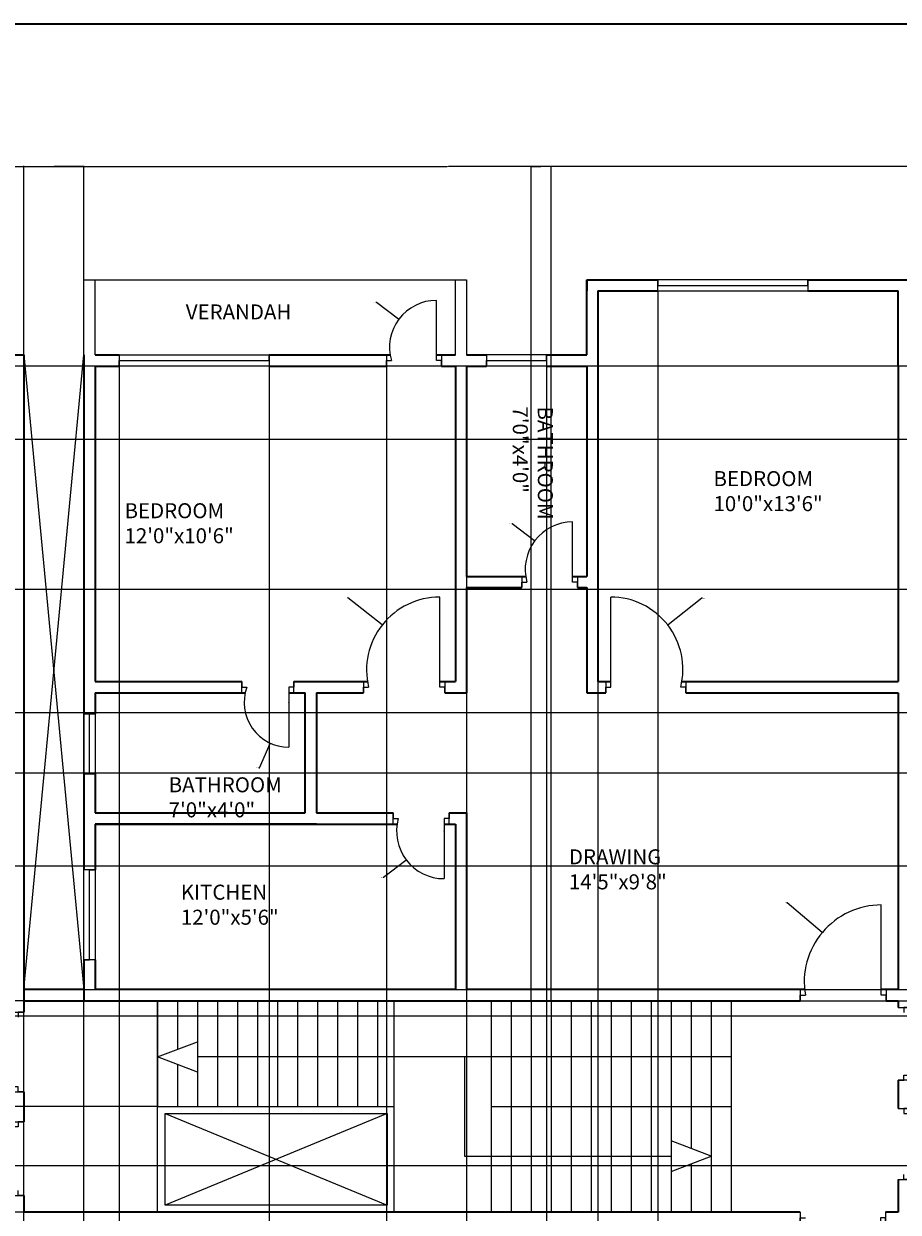
# Model space of a CAD drawing. Units: inches. Extents: x 1831 to 2867, y 1605 to 2524.
# Tile 5 of 7: x 2172 to 2522, y 2049 to 2524. Entities that reach past the tile are written whole.
import ezdxf

# ---------------------------------------------------------------- set-up
doc = ezdxf.new("R2010")
doc.units = ezdxf.units.IN
for name, color, linetype, lineweight in [('A-ANNO-DIMS', 2, 'Continuous', 18), ('A-ANNO-SYMB', 81, 'Continuous', 18), ('A-ANNO-TTLB', 7, 'Continuous', 35), ('A-AREA-IDEN', 7, 'Continuous', 18), ('A-DOOR', 11, 'Continuous', 18), ('A-FLOR-BALC', 7, 'Continuous', 25), ('A-FLOR-OPEN', 7, 'Continuous', 13), ('A-FLOR-STRS', 81, 'Continuous', 18), ('A-GLAZ', 121, 'Continuous', 18), ('A-WALL', 7, 'Continuous', 35)]:
    doc.layers.add(name, color=color, linetype=linetype, lineweight=lineweight)
doc.styles.get("Standard").update_dxf_attribs({"font": 'arial.ttf'})
doc.dimstyles.get("Standard").update_dxf_attribs({"dimtxt": 0.18, "dimasz": 0.18, "dimexe": 0.18, "dimexo": 0.0625, "dimgap": 0.09, "dimtad": 0, "dimtih": 1, "dimtoh": 1, "dimdec": 4, "dimzin": 0, "dimdsep": 46, "dimtxsty": 'Standard', "dimcen": 0.09, "dimadec": 0, "dimazin": 0, "dimtfac": 1, "dimtdec": 4, "dimtofl": 0, "dimtmove": 0, "dimatfit": 3, "dimfxl": 1, "dimtolj": 1, "dimtzin": 0, "dimarcsym": 0})

# ---------------------------------------------------------------- blocks, each defined once
blk = doc.blocks.new('WIN-60IN')
for p, q in [((4.5, 60), (0, 60)), ((0, 60), (2.25, 60)), ((0, 0), (0, 60)), ((2.25, 60), (2.25, 0)), ((4.5, 60), (4.5, 0)), ((4.5, 0), (0, 0)), ((2.25, 0), (4.5, 0))]:
    blk.add_line(p, q)
blk = doc.blocks.new('WIN-24IN')
for p, q in [((4.5, 24), (0, 24)), ((0, 24), (2.25, 24)), ((0, 0), (0, 24)), ((2.25, 24), (2.25, 0)), ((4.5, 0), (4.5, 24)), ((4.5, 0), (0, 0)), ((2.25, 0), (4.5, 0))]:
    blk.add_line(p, q)
blk = doc.blocks.new('WIN-36IN')
for p, q in [((0, 0), (0, 4.5)), ((36, 4.5), (0, 4.5)), ((36, 2.25), (0, 2.25)), ((0, 2.25), (0, 0)), ((36, 0), (36, 4.5)), ((36, 4.5), (36, 2.25)), ((0, 0), (36, 0))]:
    blk.add_line(p, q)
blk = doc.blocks.new('WIN-60IN-ALT')
for p, q in [((0, 0), (0, 4.5)), ((0, 4.5), (0, 2.25)), ((60, 4.5), (0, 4.5)), ((0, 2.25), (60, 2.25)), ((0, 0), (60, 0)), ((60, 2.25), (60, 4.5)), ((60, 4.5), (60, 0))]:
    blk.add_line(p, q)
blk = doc.blocks.new('DOOR-LEAF-36IN')
for p, q in [((0, 2), (4.5, 2)), ((4.5, 2), (2.25, 2)), ((2.25, 2), (2.25, 0)), ((2.25, 0), (38.25, 0))]:
    blk.add_line(p, q)
blk = doc.blocks.new('DOOR-LEAF-36IN-ALT')
for p, q in [((36, 2), (0, 2)), ((33.75, 0), (38.25, 0)), ((36, 0), (36, 2)), ((38.25, 0), (36, 0))]:
    blk.add_line(p, q)
blk = doc.blocks.new('DOOR-LEAF-24IN-ALT')
for p, q in [((24, 2), (0, 2)), ((21.75, 0), (26.25, 0)), ((24, 0), (24, 2)), ((26.25, 0), (24, 0))]:
    blk.add_line(p, q)
blk = doc.blocks.new('DOOR-STRIKE-JAMB')
for p, q in [((0, 0), (4.5, 0)), ((2.25, 0), (2.25, 2)), ((4.5, 0), (2.25, 0))]:
    blk.add_line(p, q)
blk = doc.blocks.new('*D22')
at = {"layer": 'A-ANNO-DIMS', "color": 0, "lineweight": -2, "transparency": 16777216}
for p, q in [((1890.05, 2218.24), (1890.05, 2467.15)), ((1890.23, 2466.97), (2341.22, 2466.97)), ((2792.79, 2466.97), (2341.8, 2466.97)), ((2792.97, 2421.74), (2792.97, 2467.15))]:
    blk.add_line(p, q, dxfattribs=at)
at = {"layer": 'A-ANNO-DIMS', "color": 0, "transparency": 16777216}
for points in [[(1890.23, 2467), (1890.23, 2466.94), (1890.05, 2466.97)], [(2792.79, 2467), (2792.79, 2466.94), (2792.97, 2466.97)]]:
    blk.add_solid(points, dxfattribs=at)
at = {"layer": 'Defpoints', "color": 0, "transparency": 16777216}
for p in [(2792.97, 2466.97), (2792.97, 2421.67), (1890.05, 2218.17)]:
    blk.add_point(p, dxfattribs=at)
at = {"layer": 'A-ANNO-DIMS', "color": 0, "transparency": 16777216, "insert": (2341.51, 2466.97), "char_height": 0.18, "attachment_point": 5}
blk.add_mtext('\\A1;903', dxfattribs=at)
blk = doc.blocks.new('*D41')
at = {"layer": 'A-ANNO-DIMS', "color": 0, "lineweight": -2, "transparency": 16777216}
for p, q in [((2156.64, 2387.11), (2156.64, 1715.69)), ((2210.17, 2387.11), (2210.17, 1715.69)), ((2156.82, 1715.87), (2183.01, 1715.87)), ((2209.99, 1715.87), (2183.8, 1715.87))]:
    blk.add_line(p, q, dxfattribs=at)
at = {"layer": 'A-ANNO-DIMS', "color": 0, "transparency": 16777216}
for points in [[(2156.82, 1715.9), (2156.82, 1715.84), (2156.64, 1715.87)], [(2209.99, 1715.9), (2209.99, 1715.84), (2210.17, 1715.87)]]:
    blk.add_solid(points, dxfattribs=at)
at = {"layer": 'Defpoints', "color": 0, "transparency": 16777216}
for p in [(2156.64, 2387.17), (2210.17, 2387.17), (2210.17, 1715.87)]:
    blk.add_point(p, dxfattribs=at)
at = {"layer": 'A-ANNO-DIMS', "color": 0, "transparency": 16777216, "insert": (2183.4, 1715.87), "char_height": 0.18, "attachment_point": 5}
blk.add_mtext('\\A1;53.52', dxfattribs=at)
blk = doc.blocks.new('*D42')
at = {"layer": 'A-ANNO-DIMS', "color": 0, "lineweight": -2, "transparency": 16777216}
for p, q in [((2270.17, 2391.61), (2270.17, 1715.69)), ((2316.97, 2391.61), (2316.97, 1715.69)), ((2270.35, 1715.87), (2293.1, 1715.87)), ((2316.79, 1715.87), (2294.04, 1715.87))]:
    blk.add_line(p, q, dxfattribs=at)
at = {"layer": 'A-ANNO-DIMS', "color": 0, "transparency": 16777216}
for points in [[(2270.35, 1715.9), (2270.35, 1715.84), (2270.17, 1715.87)], [(2316.79, 1715.9), (2316.79, 1715.84), (2316.97, 1715.87)]]:
    blk.add_solid(points, dxfattribs=at)
at = {"layer": 'Defpoints', "color": 0, "transparency": 16777216}
for p in [(2270.17, 2391.67), (2316.97, 2391.67), (2316.97, 1715.87)]:
    blk.add_point(p, dxfattribs=at)
at = {"layer": 'A-ANNO-DIMS', "color": 0, "transparency": 16777216, "insert": (2293.57, 1715.87), "char_height": 0.18, "attachment_point": 5}
blk.add_mtext('\\A1;46.805', dxfattribs=at)
blk = doc.blocks.new('*D43')
at = {"layer": 'A-ANNO-DIMS', "color": 0, "lineweight": -2, "transparency": 16777216}
for p, q in [((2349.05, 2387.11), (2349.05, 1715.69)), ((2381.01, 2387.11), (2381.01, 1715.69)), ((2349.23, 1715.87), (2364.57, 1715.87)), ((2380.83, 1715.87), (2365.49, 1715.87))]:
    blk.add_line(p, q, dxfattribs=at)
at = {"layer": 'A-ANNO-DIMS', "color": 0, "transparency": 16777216}
for points in [[(2349.23, 1715.9), (2349.23, 1715.84), (2349.05, 1715.87)], [(2380.83, 1715.9), (2380.83, 1715.84), (2381.01, 1715.87)]]:
    blk.add_solid(points, dxfattribs=at)
at = {"layer": 'Defpoints', "color": 0, "transparency": 16777216}
for p in [(2349.05, 2387.17), (2381.01, 2387.17), (2381.01, 1715.87)]:
    blk.add_point(p, dxfattribs=at)
at = {"layer": 'A-ANNO-DIMS', "color": 0, "transparency": 16777216, "insert": (2365.03, 1715.87), "char_height": 0.18, "attachment_point": 5}
blk.add_mtext('\\A1;31.956', dxfattribs=at)
blk = doc.blocks.new('*D44')
at = {"layer": 'A-ANNO-DIMS', "color": 0, "lineweight": -2, "transparency": 16777216}
for p, q in [((2401.55, 2417.11), (2401.55, 1715.69)), ((2425.47, 2417.11), (2425.47, 1715.69)), ((2401.73, 1715.87), (2413.05, 1715.87)), ((2425.29, 1715.87), (2413.98, 1715.87))]:
    blk.add_line(p, q, dxfattribs=at)
at = {"layer": 'A-ANNO-DIMS', "color": 0, "transparency": 16777216}
for points in [[(2401.73, 1715.9), (2401.73, 1715.84), (2401.55, 1715.87)], [(2425.29, 1715.9), (2425.29, 1715.84), (2425.47, 1715.87)]]:
    blk.add_solid(points, dxfattribs=at)
at = {"layer": 'Defpoints', "color": 0, "transparency": 16777216}
for p in [(2401.55, 2417.17), (2425.47, 2417.17), (2425.47, 1715.87)]:
    blk.add_point(p, dxfattribs=at)
at = {"layer": 'A-ANNO-DIMS', "color": 0, "transparency": 16777216, "insert": (2413.51, 1715.87), "char_height": 0.18, "attachment_point": 5}
blk.add_mtext('\\A1;23.924', dxfattribs=at)
blk = doc.blocks.new('*D49')
at = {"layer": 'A-ANNO-DIMS', "color": 0, "lineweight": -2, "transparency": 16777216}
for p, q in [((2786.99, 2387.17), (1844.57, 2387.17)), ((1844.75, 2386.99), (1844.75, 2372.7)), ((1844.75, 2358.05), (1844.75, 2372.34)), ((2786.99, 2357.87), (1844.57, 2357.87))]:
    blk.add_line(p, q, dxfattribs=at)
at = {"layer": 'A-ANNO-DIMS', "color": 0, "transparency": 16777216}
for points in [[(1844.72, 2386.99), (1844.78, 2386.99), (1844.75, 2387.17)], [(1844.72, 2358.05), (1844.78, 2358.05), (1844.75, 2357.87)]]:
    blk.add_solid(points, dxfattribs=at)
at = {"layer": 'Defpoints', "color": 0, "transparency": 16777216}
for p in [(2787.05, 2387.17), (1844.75, 2357.87), (2787.05, 2357.87)]:
    blk.add_point(p, dxfattribs=at)
at = {"layer": 'A-ANNO-DIMS', "color": 0, "transparency": 16777216, "insert": (1844.75, 2372.52), "char_height": 0.18, "attachment_point": 5}
blk.add_mtext('\\A1;29.31', dxfattribs=at)
blk = doc.blocks.new('*D50')
at = {"layer": 'A-ANNO-DIMS', "color": 0, "lineweight": -2, "transparency": 16777216}
for p, q in [((2786.99, 2297.87), (1844.57, 2297.87)), ((1844.75, 2297.69), (1844.75, 2273.42)), ((1844.75, 2248.78), (1844.75, 2273.05)), ((2786.99, 2248.6), (1844.57, 2248.6))]:
    blk.add_line(p, q, dxfattribs=at)
at = {"layer": 'A-ANNO-DIMS', "color": 0, "transparency": 16777216}
for points in [[(1844.72, 2297.69), (1844.78, 2297.69), (1844.75, 2297.87)], [(1844.72, 2248.78), (1844.78, 2248.78), (1844.75, 2248.6)]]:
    blk.add_solid(points, dxfattribs=at)
at = {"layer": 'Defpoints', "color": 0, "transparency": 16777216}
for p in [(2787.05, 2297.87), (1844.75, 2248.6), (2787.05, 2248.6)]:
    blk.add_point(p, dxfattribs=at)
at = {"layer": 'A-ANNO-DIMS', "color": 0, "transparency": 16777216, "insert": (1844.75, 2273.23), "char_height": 0.18, "attachment_point": 5}
blk.add_mtext('\\A1;49.26', dxfattribs=at)
blk = doc.blocks.new('*D51')
at = {"layer": 'A-ANNO-DIMS', "color": 0, "lineweight": -2, "transparency": 16777216}
for p, q in [((2786.99, 2224.6), (1844.57, 2224.6)), ((1844.75, 2224.42), (1844.75, 2206.21)), ((1844.75, 2187.63), (1844.75, 2205.85)), ((2786.99, 2187.45), (1844.57, 2187.45))]:
    blk.add_line(p, q, dxfattribs=at)
at = {"layer": 'A-ANNO-DIMS', "color": 0, "transparency": 16777216}
for points in [[(1844.72, 2224.42), (1844.78, 2224.42), (1844.75, 2224.6)], [(1844.72, 2187.63), (1844.78, 2187.63), (1844.75, 2187.45)]]:
    blk.add_solid(points, dxfattribs=at)
at = {"layer": 'Defpoints', "color": 0, "transparency": 16777216}
for p in [(2787.05, 2224.6), (1844.75, 2187.45), (2787.05, 2187.45)]:
    blk.add_point(p, dxfattribs=at)
at = {"layer": 'A-ANNO-DIMS', "color": 0, "transparency": 16777216, "insert": (1844.75, 2206.03), "char_height": 0.18, "attachment_point": 5}
blk.add_mtext('\\A1;37.15', dxfattribs=at)
blk = doc.blocks.new('*D52')
at = {"layer": 'A-ANNO-DIMS', "color": 0, "lineweight": -2, "transparency": 16777216}
for p, q in [((2786.99, 2127.45), (1844.57, 2127.45)), ((1844.75, 2127.27), (1844.75, 2097.76)), ((1844.75, 2067.88), (1844.75, 2097.39)), ((2786.99, 2067.7), (1844.57, 2067.7))]:
    blk.add_line(p, q, dxfattribs=at)
at = {"layer": 'A-ANNO-DIMS', "color": 0, "transparency": 16777216}
for points in [[(1844.72, 2127.27), (1844.78, 2127.27), (1844.75, 2127.45)], [(1844.72, 2067.88), (1844.78, 2067.88), (1844.75, 2067.7)]]:
    blk.add_solid(points, dxfattribs=at)
at = {"layer": 'Defpoints', "color": 0, "transparency": 16777216}
for p in [(2787.05, 2127.45), (1844.75, 2067.7), (2787.05, 2067.7)]:
    blk.add_point(p, dxfattribs=at)
at = {"layer": 'A-ANNO-DIMS', "color": 0, "transparency": 16777216, "insert": (1844.75, 2097.57), "char_height": 0.18, "attachment_point": 5}
blk.add_mtext('\\A1;59.76', dxfattribs=at)
blk = doc.blocks.new('*D60')
at = {"layer": 'A-ANNO-DIMS', "color": 0, "lineweight": -2, "transparency": 16777216}
for p, q in [((2225.43, 2091.42), (1844.57, 2091.42)), ((1844.75, 2091.24), (1844.75, 2070.48)), ((1844.75, 2049.35), (1844.75, 2070.12)), ((2225.43, 2049.17), (1844.57, 2049.17))]:
    blk.add_line(p, q, dxfattribs=at)
at = {"layer": 'A-ANNO-DIMS', "color": 0, "transparency": 16777216}
for points in [[(1844.72, 2091.24), (1844.78, 2091.24), (1844.75, 2091.42)], [(1844.72, 2049.35), (1844.78, 2049.35), (1844.75, 2049.17)]]:
    blk.add_solid(points, dxfattribs=at)
at = {"layer": 'Defpoints', "color": 0, "transparency": 16777216}
for p in [(1844.75, 2091.42), (2225.49, 2091.42), (2225.49, 2049.17)]:
    blk.add_point(p, dxfattribs=at)
at = {"layer": 'A-ANNO-DIMS', "color": 0, "transparency": 16777216, "insert": (1844.75, 2070.3), "char_height": 0.18, "attachment_point": 5}
blk.add_mtext('\\A1;42.25', dxfattribs=at)
blk = doc.blocks.new('*D61')
at = {"layer": 'A-ANNO-DIMS', "color": 0, "lineweight": -2, "transparency": 16777216}
for p, q in [((2225.43, 2133.67), (1844.57, 2133.67)), ((1844.75, 2133.49), (1844.75, 2112.73)), ((1844.75, 2091.6), (1844.75, 2112.37)), ((2225.43, 2091.42), (1844.57, 2091.42))]:
    blk.add_line(p, q, dxfattribs=at)
at = {"layer": 'A-ANNO-DIMS', "color": 0, "transparency": 16777216}
for points in [[(1844.72, 2133.49), (1844.78, 2133.49), (1844.75, 2133.67)], [(1844.72, 2091.6), (1844.78, 2091.6), (1844.75, 2091.42)]]:
    blk.add_solid(points, dxfattribs=at)
at = {"layer": 'Defpoints', "color": 0, "transparency": 16777216}
for p in [(1844.75, 2133.67), (2225.49, 2133.67), (2225.49, 2091.42)]:
    blk.add_point(p, dxfattribs=at)
at = {"layer": 'A-ANNO-DIMS', "color": 0, "transparency": 16777216, "insert": (1844.75, 2112.55), "char_height": 0.18, "attachment_point": 5}
blk.add_mtext('\\A1;42.25', dxfattribs=at)
blk = doc.blocks.new('*D62')
at = {"layer": 'A-ANNO-DIMS', "color": 0, "lineweight": -2, "transparency": 16777216}
for p, q in [((2374.81, 2133.74), (2374.81, 2467.15)), ((2374.99, 2466.97), (2378.66, 2466.97)), ((2382.63, 2466.97), (2378.95, 2466.97)), ((2382.81, 2133.74), (2382.81, 2467.15))]:
    blk.add_line(p, q, dxfattribs=at)
at = {"layer": 'A-ANNO-DIMS', "color": 0, "transparency": 16777216}
for points in [[(2374.99, 2467), (2374.99, 2466.94), (2374.81, 2466.97)], [(2382.63, 2467), (2382.63, 2466.94), (2382.81, 2466.97)]]:
    blk.add_solid(points, dxfattribs=at)
at = {"layer": 'Defpoints', "color": 0, "transparency": 16777216}
for p in [(2382.81, 2466.97), (2374.81, 2133.67), (2382.81, 2133.67)]:
    blk.add_point(p, dxfattribs=at)
at = {"layer": 'A-ANNO-DIMS', "color": 0, "transparency": 16777216, "insert": (2378.81, 2466.97), "char_height": 0.18, "attachment_point": 5}
blk.add_mtext('\\A1;8', dxfattribs=at)
blk = doc.blocks.new('*D63')
at = {"layer": 'A-ANNO-DIMS', "color": 0, "lineweight": -2, "transparency": 16777216}
for p, q in [((2172.05, 1795.74), (2172.05, 2467.15)), ((2172.23, 2466.97), (2183.83, 2466.97)), ((2195.87, 2466.97), (2184.27, 2466.97)), ((2196.05, 1795.74), (2196.05, 2467.15))]:
    blk.add_line(p, q, dxfattribs=at)
at = {"layer": 'A-ANNO-DIMS', "color": 0, "transparency": 16777216}
for points in [[(2172.23, 2467), (2172.23, 2466.94), (2172.05, 2466.97)], [(2195.87, 2467), (2195.87, 2466.94), (2196.05, 2466.97)]]:
    blk.add_solid(points, dxfattribs=at)
at = {"layer": 'Defpoints', "color": 0, "transparency": 16777216}
for p in [(2196.05, 2466.97), (2172.05, 1795.67), (2196.05, 1795.67)]:
    blk.add_point(p, dxfattribs=at)
at = {"layer": 'A-ANNO-DIMS', "color": 0, "transparency": 16777216, "insert": (2184.05, 2466.97), "char_height": 0.18, "attachment_point": 5}
blk.add_mtext('\\A1;24', dxfattribs=at)
blk = doc.blocks.new('*D64')
at = {"layer": 'A-ANNO-DIMS', "color": 0, "lineweight": -2, "transparency": 16777216}
for p, q in [((2172.11, 2138.17), (2838.45, 2138.17)), ((2838.27, 2137.99), (2838.27, 2136.11)), ((2172.11, 2133.67), (2838.45, 2133.67)), ((2838.27, 2133.85), (2838.27, 2135.74))]:
    blk.add_line(p, q, dxfattribs=at)
at = {"layer": 'A-ANNO-DIMS', "color": 0, "transparency": 16777216}
for points in [[(2838.24, 2137.99), (2838.3, 2137.99), (2838.27, 2138.17)], [(2838.24, 2133.85), (2838.3, 2133.85), (2838.27, 2133.67)]]:
    blk.add_solid(points, dxfattribs=at)
at = {"layer": 'Defpoints', "color": 0, "transparency": 16777216}
for p in [(2172.05, 2138.17), (2172.05, 2133.67), (2838.27, 2133.67)]:
    blk.add_point(p, dxfattribs=at)
at = {"layer": 'A-ANNO-DIMS', "color": 0, "transparency": 16777216, "insert": (2838.27, 2135.92), "char_height": 0.18, "attachment_point": 5}
blk.add_mtext('\\A1;4.5', dxfattribs=at)
blk = doc.blocks.new('*D65')
at = {"layer": 'A-ANNO-DIMS', "color": 0, "lineweight": -2, "transparency": 16777216}
for p, q in [((2476.93, 2172.9), (2477.11, 2172.9)), ((2477.11, 2172.9), (2491.1, 2161.1)), ((2514.7, 2141.11), (2514.88, 2141.11)), ((2514.79, 2141.02), (2514.79, 2141.2))]:
    blk.add_line(p, q, dxfattribs=at)
at = {"layer": 'A-ANNO-DIMS', "color": 0, "transparency": 16777216}
blk.add_solid([(2491.12, 2161.12), (2491.08, 2161.07), (2491.24, 2160.98)], dxfattribs=at)
at = {"layer": 'Defpoints', "color": 0, "transparency": 16777216}
for p in [(2491.24, 2160.98), (2514.79, 2141.11)]:
    blk.add_point(p, dxfattribs=at)
at = {"layer": 'A-ANNO-DIMS', "color": 0, "transparency": 16777216, "insert": (2476.47, 2172.9), "char_height": 0.18, "attachment_point": 5}
blk.add_mtext('\\A1;R30.81', dxfattribs=at)
blk = doc.blocks.new('*D68')
at = {"layer": 'A-ANNO-DIMS', "color": 0, "lineweight": -2, "transparency": 16777216}
for p, q in [((2301.42, 2294.71), (2301.6, 2294.71)), ((2301.6, 2294.71), (2315.23, 2283.93)), ((2338.24, 2265.65), (2338.42, 2265.65)), ((2338.33, 2265.56), (2338.33, 2265.74))]:
    blk.add_line(p, q, dxfattribs=at)
at = {"layer": 'A-ANNO-DIMS', "color": 0, "transparency": 16777216}
blk.add_solid([(2315.25, 2283.95), (2315.21, 2283.9), (2315.37, 2283.82)], dxfattribs=at)
at = {"layer": 'Defpoints', "color": 0, "transparency": 16777216}
for p in [(2315.37, 2283.82), (2338.33, 2265.65)]:
    blk.add_point(p, dxfattribs=at)
at = {"layer": 'A-ANNO-DIMS', "color": 0, "transparency": 16777216, "insert": (2300.94, 2294.71), "char_height": 0.18, "attachment_point": 5}
blk.add_mtext('\\A1;R29.27', dxfattribs=at)
blk = doc.blocks.new('*D69')
at = {"layer": 'A-ANNO-DIMS', "color": 0, "lineweight": -2, "transparency": 16777216}
for p, q in [((2443.11, 2294.41), (2429.57, 2283.88)), ((2443.29, 2294.41), (2443.11, 2294.41)), ((2406.53, 2266.03), (2406.71, 2266.03)), ((2406.62, 2265.94), (2406.62, 2266.12))]:
    blk.add_line(p, q, dxfattribs=at)
at = {"layer": 'A-ANNO-DIMS', "color": 0, "transparency": 16777216}
blk.add_solid([(2429.55, 2283.91), (2429.59, 2283.86), (2429.43, 2283.77)], dxfattribs=at)
at = {"layer": 'Defpoints', "color": 0, "transparency": 16777216}
for p in [(2429.43, 2283.77), (2406.62, 2266.03)]:
    blk.add_point(p, dxfattribs=at)
at = {"layer": 'A-ANNO-DIMS', "color": 0, "transparency": 16777216, "insert": (2443.77, 2294.41), "char_height": 0.18, "attachment_point": 5}
blk.add_mtext('\\A1;R28.89', dxfattribs=at)
blk = doc.blocks.new('*D89')
at = {"layer": 'A-ANNO-DIMS', "color": 0, "lineweight": -2, "transparency": 16777216}
for p, q in [((2339.96, 2201.43), (2340.14, 2201.43)), ((2340.05, 2201.34), (2340.05, 2201.52)), ((2315.89, 2182.97), (2324.81, 2189.78)), ((2315.71, 2182.97), (2315.89, 2182.97))]:
    blk.add_line(p, q, dxfattribs=at)
at = {"layer": 'A-ANNO-DIMS', "color": 0, "transparency": 16777216}
blk.add_solid([(2324.79, 2189.81), (2324.82, 2189.76), (2324.95, 2189.89)], dxfattribs=at)
at = {"layer": 'Defpoints', "color": 0, "transparency": 16777216}
for p in [(2340.05, 2201.43), (2324.95, 2189.89)]:
    blk.add_point(p, dxfattribs=at)
at = {"layer": 'A-ANNO-DIMS', "color": 0, "transparency": 16777216, "insert": (2315.16, 2182.97), "char_height": 0.18, "attachment_point": 5}
blk.add_mtext('\\A1;R19.004', dxfattribs=at)
blk = doc.blocks.new('*D91')
at = {"layer": 'A-ANNO-DIMS', "color": 0, "lineweight": -2, "transparency": 16777216}
for p, q in [((2367.09, 2324.31), (2367.27, 2324.31)), ((2367.27, 2324.31), (2376.17, 2317.56)), ((2391.29, 2306), (2391.47, 2306)), ((2391.38, 2305.91), (2391.38, 2306.09))]:
    blk.add_line(p, q, dxfattribs=at)
at = {"layer": 'A-ANNO-DIMS', "color": 0, "transparency": 16777216}
blk.add_solid([(2376.19, 2317.58), (2376.15, 2317.53), (2376.31, 2317.45)], dxfattribs=at)
at = {"layer": 'Defpoints', "color": 0, "transparency": 16777216}
for p in [(2376.31, 2317.45), (2391.38, 2306)]:
    blk.add_point(p, dxfattribs=at)
at = {"layer": 'A-ANNO-DIMS', "color": 0, "transparency": 16777216, "insert": (2366.54, 2324.31), "char_height": 0.18, "attachment_point": 5}
blk.add_mtext('\\A1;R18.923', dxfattribs=at)
blk = doc.blocks.new('*D92')
at = {"layer": 'A-ANNO-DIMS', "color": 0, "lineweight": -2, "transparency": 16777216}
for p, q in [((2312.8, 2412.69), (2312.98, 2412.69)), ((2312.98, 2412.69), (2321.84, 2406.03)), ((2336.9, 2394.66), (2337.08, 2394.66)), ((2336.99, 2394.57), (2336.99, 2394.75))]:
    blk.add_line(p, q, dxfattribs=at)
at = {"layer": 'A-ANNO-DIMS', "color": 0, "transparency": 16777216}
blk.add_solid([(2321.86, 2406.06), (2321.82, 2406.01), (2321.99, 2405.93)], dxfattribs=at)
at = {"layer": 'Defpoints', "color": 0, "transparency": 16777216}
for p in [(2321.99, 2405.93), (2336.99, 2394.66)]:
    blk.add_point(p, dxfattribs=at)
at = {"layer": 'A-ANNO-DIMS', "color": 0, "transparency": 16777216, "insert": (2312.25, 2412.69), "char_height": 0.18, "attachment_point": 5}
blk.add_mtext('\\A1;R18.767', dxfattribs=at)
blk = doc.blocks.new('*D104')
at = {"layer": 'A-ANNO-DIMS', "color": 0, "lineweight": -2, "transparency": 16777216}
for p, q in [((2277.96, 2252.84), (2278.14, 2252.84)), ((2278.05, 2252.75), (2278.05, 2252.93)), ((2266.21, 2226.74), (2270.57, 2236.36)), ((2266.03, 2226.74), (2266.21, 2226.74))]:
    blk.add_line(p, q, dxfattribs=at)
at = {"layer": 'A-ANNO-DIMS', "color": 0, "transparency": 16777216}
blk.add_solid([(2270.55, 2236.37), (2270.6, 2236.35), (2270.65, 2236.53)], dxfattribs=at)
at = {"layer": 'Defpoints', "color": 0, "transparency": 16777216}
for p in [(2278.05, 2252.84), (2270.65, 2236.53)]:
    blk.add_point(p, dxfattribs=at)
at = {"layer": 'A-ANNO-DIMS', "color": 0, "transparency": 16777216, "insert": (2265.48, 2226.74), "char_height": 0.18, "attachment_point": 5}
blk.add_mtext('\\A1;R17.915', dxfattribs=at)

msp = doc.modelspace()

# ---------------------------------------------------------------- linework, layer by layer
at = {"layer": 'A-ANNO-SYMB'}
for p, q in [((2225.4925, 2111.2442), (2241.4925, 2117.2005)), ((2241.4925, 2117.2005), (2241.4925, 2105.1583)), ((2241.4925, 2105.1583), (2225.4925, 2111.2442)), ((2454.8055, 2111.2442), (2241.4925, 2111.2442)), ((2348.149, 2111.2442), (2348.149, 2071.6055)), ((2446.8055, 2071.6055), (2430.8055, 2077.7473)), ((2430.8055, 2077.7473), (2430.8055, 2065.4193)), ((2348.149, 2071.6055), (2430.8055, 2071.6055)), ((2430.8055, 2065.4193), (2446.8055, 2071.6055))]:
    msp.add_line(p, q, dxfattribs=at)
at = {"layer": 'A-ANNO-TTLB'}
msp.add_lwpolyline([(1831.1248, 2523.9204), (2867.0416, 2523.9204), (2867.0416, 1605.0781), (1831.1248, 1605.0781)], close=True, dxfattribs=at)
at = {"layer": 'A-DOOR'}
for centre, radius, start, end in [((2336.9932, 2394.6565), 18.7673, 90, 196.189982), ((2391.3796, 2306.0013), 18.9225, 90, 195.564932), ((2338.3265, 2265.6546), 29.2692, 90, 193.29495), ((2406.6247, 2266.0321), 28.8917, 345.757123, 90), ((2278.0539, 2252.8387), 17.9149, 160.143485, 270), ((2340.0513, 2201.4282), 19.0045, 164.760076, 270), ((2514.791, 2141.1122), 30.8116, 90, 189.694325)]:
    msp.add_arc(centre, radius, start, end, dxfattribs=at)
at = {"layer": 'A-FLOR-BALC'}
for p, q in [((2196.051, 2391.6738), (2196.051, 2421.6738)), ((2196.051, 2421.6738), (2349.051, 2421.6738)), ((2200.551, 2391.6738), (2200.551, 2421.6738)), ((2344.551, 2391.6738), (2344.551, 2421.6738)), ((2349.051, 2421.6738), (2349.051, 2409.6738)), ((2196.051, 2391.6738), (2196.051, 2409.6738)), ((2349.051, 2409.6738), (2349.051, 2391.6738))]:
    msp.add_line(p, q, dxfattribs=at)
at = {"layer": 'A-FLOR-OPEN'}
for p, q in [((2172.051, 2138.1738), (2196.051, 2391.6738)), ((2172.051, 2391.6738), (2196.051, 2138.1738)), ((2317.3176, 2088.5621), (2228.5133, 2052.0199)), ((2228.5133, 2088.5621), (2317.3176, 2052.0199))]:
    msp.add_line(p, q, dxfattribs=at)
msp.add_lwpolyline([(2228.5133, 2088.5621), (2317.3176, 2088.5621), (2317.3176, 2052.0199), (2228.5133, 2052.0199)], close=True, dxfattribs=at)
at = {"layer": 'A-FLOR-STRS'}
for p, q in [((2225.4925, 2049.1738), (2225.4925, 2133.6738)), ((2225.4925, 2133.6738), (2225.4925, 2091.4238)), ((2233.4925, 2133.6738), (2233.4925, 2114.2223)), ((2241.4925, 2133.6738), (2241.4925, 2091.4238)), ((2249.4925, 2133.6738), (2249.4925, 2091.4238)), ((2257.4925, 2133.6738), (2257.4925, 2091.4238)), ((2265.4925, 2133.6738), (2265.4925, 2091.4238)), ((2273.4925, 2133.6738), (2273.4925, 2091.4238)), ((2281.4925, 2133.6738), (2281.4925, 2091.4238)), ((2289.4925, 2133.6738), (2289.4925, 2091.4238)), ((2297.4925, 2133.6738), (2297.4925, 2091.4238)), ((2305.4925, 2133.6738), (2305.4925, 2091.4238)), ((2313.4925, 2133.6738), (2313.4925, 2091.4238)), ((2319.9867, 2133.6738), (2319.9867, 2049.1738)), ((2358.8055, 2133.6738), (2358.8055, 2049.1738)), ((2366.8055, 2133.6738), (2366.8055, 2049.1738)), ((2374.8055, 2133.6738), (2374.8055, 2049.1738)), ((2382.8055, 2133.6738), (2382.8055, 2049.1738)), ((2390.8055, 2133.6738), (2390.8055, 2049.1738)), ((2398.8055, 2133.6738), (2398.8055, 2049.1738)), ((2406.8055, 2133.6738), (2406.8055, 2049.1738)), ((2414.8055, 2133.6738), (2414.8055, 2049.1738)), ((2422.8055, 2133.6738), (2422.8055, 2049.1738)), ((2430.8055, 2133.6738), (2430.8055, 2049.1738)), ((2438.8055, 2133.6738), (2438.8055, 2074.6764)), ((2446.8055, 2133.6738), (2446.8055, 2049.1738)), ((2454.8055, 2133.6738), (2454.8055, 2049.1738)), ((2233.4925, 2108.2012), (2233.4925, 2091.4238)), ((2225.4925, 2091.4238), (2319.9867, 2091.4238)), ((2358.8055, 2091.4238), (2454.8055, 2091.4238)), ((2438.8055, 2068.5124), (2438.8055, 2049.1738))]:
    msp.add_line(p, q, dxfattribs=at)
at = {"layer": 'A-GLAZ'}
for p, q in [((2196.051, 2248.2739), (2199.5432, 2248.2739)), ((2196.051, 2248.2739), (2196.051, 2224.2739)), ((2199.5432, 2248.2739), (2197.7971, 2248.2739)), ((2198.6701, 2248.2739), (2198.1796, 2248.2739)), ((2198.1796, 2248.2739), (2198.1796, 2224.2739)), ((2200.551, 2248.2739), (2198.6701, 2248.2739)), ((2199.5432, 2248.2739), (2200.551, 2248.2739)), ((2200.551, 2248.2739), (2200.551, 2224.2739)), ((2198.1796, 2224.2739), (2196.051, 2224.2739)), ((2196.051, 2224.2739), (2200.551, 2224.2739))]:
    msp.add_line(p, q, dxfattribs=at)
at = {"layer": 'A-WALL'}
for p, q in [((2397.051, 2391.6738), (2397.051, 2421.6738)), ((2397.051, 2421.6738), (2425.4746, 2421.6738)), ((2397.051, 2421.6738), (2397.051, 2417.1738)), ((2485.4746, 2421.6738), (2526.051, 2421.6738)), ((2401.551, 2417.1738), (2401.551, 2387.1738)), ((2401.551, 2417.1738), (2425.4746, 2417.1738)), ((2485.4746, 2417.1738), (2521.551, 2417.1738)), ((2521.551, 2387.1738), (2521.551, 2417.1738)), ((2156.6429, 2391.6738), (2172.051, 2391.6738)), ((2172.051, 2391.6738), (2172.051, 2129.1206)), ((2196.051, 2391.6738), (2196.051, 2248.2739)), ((2200.551, 2391.6738), (2210.1653, 2391.6738)), ((2270.1653, 2391.6738), (2318.4645, 2391.6738)), ((2336.9932, 2391.6738), (2344.551, 2391.6738)), ((2349.051, 2391.6738), (2357.0066, 2391.6738)), ((2381.0066, 2391.6738), (2397.051, 2391.6738)), ((2200.551, 2387.1738), (2200.551, 2261.1738)), ((2200.551, 2387.1738), (2210.1653, 2387.1738)), ((2270.1653, 2387.1738), (2316.9702, 2387.1738)), ((2338.9932, 2387.1738), (2344.551, 2387.1738)), ((2344.551, 2387.1738), (2344.551, 2261.1738)), ((2349.051, 2387.1738), (2349.051, 2303.1738)), ((2349.051, 2387.1738), (2357.0066, 2387.1738)), ((2381.0066, 2387.1738), (2397.051, 2387.1738)), ((2397.051, 2387.1738), (2397.051, 2303.1738)), ((2401.551, 2387.1738), (2401.551, 2261.1738)), ((2521.551, 2387.1738), (2521.551, 2261.1738)), ((2349.051, 2303.1738), (2372.6695, 2303.1738)), ((2391.3796, 2303.1738), (2397.051, 2303.1738)), ((2349.051, 2298.6738), (2371.151, 2298.6738)), ((2349.051, 2298.6738), (2349.051, 2256.6738)), ((2393.3796, 2298.6738), (2397.051, 2298.6738)), ((2397.051, 2298.6738), (2397.051, 2256.6738)), ((2200.551, 2261.1738), (2259.2041, 2261.1738)), ((2280.0539, 2261.1738), (2309.4023, 2261.1738)), ((2338.3265, 2261.1738), (2344.551, 2261.1738)), ((2401.551, 2261.1738), (2406.6247, 2261.1738)), ((2435.105, 2261.1738), (2521.551, 2261.1738)), ((2200.551, 2256.6738), (2260.5543, 2256.6738)), ((2200.551, 2256.6738), (2200.551, 2248.2739)), ((2200.551, 2256.6738), (2200.551, 2248.2739)), ((2278.0539, 2256.6738), (2284.551, 2256.6738)), ((2284.551, 2208.6738), (2284.551, 2256.6738)), ((2289.051, 2256.6738), (2289.051, 2208.6738)), ((2289.051, 2256.6738), (2307.8418, 2256.6738)), ((2340.3265, 2256.6738), (2344.551, 2256.6738)), ((2344.551, 2256.6738), (2349.051, 2256.6738)), ((2397.051, 2256.6738), (2404.6247, 2256.6738)), ((2436.6283, 2256.6738), (2521.551, 2256.6738)), ((2521.551, 2256.6738), (2521.551, 2138.1738)), ((2196.051, 2224.2739), (2196.051, 2186.0032)), ((2200.551, 2224.2739), (2200.551, 2208.6738)), ((2200.551, 2224.2739), (2200.551, 2208.6738)), ((2200.551, 2208.6738), (2284.551, 2208.6738)), ((2289.051, 2208.6738), (2319.7152, 2208.6738)), ((2342.0513, 2208.6738), (2349.051, 2208.6738)), ((2349.051, 2208.6738), (2349.051, 2138.1738)), ((2289.051, 2204.1738), (2200.551, 2204.1738)), ((2200.551, 2204.1738), (2321.2462, 2204.1738)), ((2200.551, 2204.1738), (2200.551, 2186.0032)), ((2340.0513, 2204.1738), (2344.551, 2204.1738)), ((2344.551, 2204.1738), (2344.551, 2138.1738)), ((2344.551, 2204.1738), (2344.551, 2138.1738)), ((2196.051, 2150.0032), (2196.051, 2133.6738)), ((2200.551, 2150.0032), (2200.551, 2138.1738)), ((2196.051, 2138.1738), (2172.051, 2138.1738)), ((2344.551, 2138.1738), (2200.551, 2138.1738)), ((2484.1198, 2138.1738), (2349.051, 2138.1738)), ((2521.551, 2138.1738), (2514.791, 2138.1738)), ((2172.051, 2133.6738), (2196.051, 2133.6738)), ((2196.051, 2133.6738), (2482.4194, 2133.6738)), ((2516.791, 2133.6738), (2521.551, 2133.6738)), ((2521.551, 2133.6738), (2521.551, 2130.9218)), ((2521.551, 2101.8924), (2521.551, 2090.5911)), ((2172.051, 2097.2455), (2172.051, 2085.2638)), ((2521.551, 2062.2002), (2521.551, 2049.1738)), ((2172.051, 2055.8862), (2172.051, 2049.1738)), ((2200.551, 2049.1738), (2172.051, 2049.1738)), ((2482.4194, 2049.1738), (2200.551, 2049.1738)), ((2482.4194, 2049.1738), (2349.051, 2049.1738)), ((2521.551, 2049.1738), (2516.4879, 2049.1738)), ((2521.551, 2049.1738), (2516.4879, 2049.1738))]:
    msp.add_line(p, q, dxfattribs=at)

# ---------------------------------------------------------------- block references
at = {"layer": 'A-DOOR', "extrusion": (0, 0, -1), "zscale": -1}
for name, p, rotation in [('DOOR-LEAF-24IN-ALT', (-2338.9932, 2413.4238), 270.0000000000013), ('DOOR-LEAF-24IN-ALT', (-2393.3796, 2324.9238), 270.0000000000001), ('DOOR-LEAF-36IN-ALT', (-2340.3265, 2294.9238), 270), ('DOOR-STRIKE-JAMB', (-2259.2041, 2256.6738), 89.99999999999876), ('DOOR-STRIKE-JAMB', (-2436.6283, 2261.1738), 270.0000000000085), ('DOOR-STRIKE-JAMB', (-2319.7152, 2204.1738), 90.00000000000854), ('DOOR-LEAF-36IN-ALT', (-2516.791, 2171.9238), 270), ('DOOR-STRIKE-JAMB', (-2167.551, 2129.1206), 180), ('DOOR-STRIKE-JAMB', (-2521.551, 2130.9218), 180), ('DOOR-LEAF-36IN-ALT', (-2133.801, 2085.2638), 180)]:
    msp.add_blockref(name, p, dxfattribs=dict(at, rotation=rotation))
at = {"layer": 'A-DOOR'}
for name, p, rotation in [('DOOR-STRIKE-JAMB', (2316.9702, 2391.6738), 269.9999999999988), ('DOOR-STRIKE-JAMB', (2371.151, 2303.1738), 269.9999999999988), ('DOOR-LEAF-36IN-ALT', (2404.6247, 2294.9238), 270), ('DOOR-LEAF-24IN-ALT', (2280.0539, 2234.9238), 90.00000000000006), ('DOOR-STRIKE-JAMB', (2307.8418, 2261.1738), 270.0000000000085), ('DOOR-LEAF-24IN-ALT', (2342.0513, 2182.4238), 90.00000000000006), ('DOOR-STRIKE-JAMB', (2482.4194, 2138.1738), 269.9999999999988), ('DOOR-STRIKE-JAMB', (2482.4194, 2049.1738), 269.9999999999957), ('DOOR-LEAF-36IN', (2514.4879, 2049.1738), 269.9999999999984)]:
    msp.add_blockref(name, p, dxfattribs=dict(at, rotation=rotation))
at = {"layer": 'A-DOOR', "extrusion": (0, 0, -1), "zscale": -1}
msp.add_blockref('DOOR-LEAF-36IN-ALT', (-2559.801, 2101.8924), dxfattribs=at)
at = {"layer": 'A-DOOR'}
for name, p in [('DOOR-LEAF-36IN-ALT', (2133.801, 2097.2455)), ('DOOR-LEAF-36IN', (2521.551, 2088.5911)), ('DOOR-STRIKE-JAMB', (2521.551, 2062.2002)), ('DOOR-STRIKE-JAMB', (2167.551, 2055.8862))]:
    msp.add_blockref(name, p, dxfattribs=at)
at = {"layer": 'A-GLAZ'}
msp.add_blockref('WIN-60IN-ALT', (2425.4746, 2417.1738), dxfattribs=at)
for name, p, rotation in [('WIN-60IN', (2270.1653, 2387.1738), 89.9999999999992), ('WIN-24IN', (2381.0066, 2387.1738), 89.99999999999726)]:
    msp.add_blockref(name, p, dxfattribs=dict(at, rotation=rotation))
at = {"layer": 'A-GLAZ', "extrusion": (0, 0, -1), "zscale": -1, "rotation": 270}
msp.add_blockref('WIN-36IN', (-2200.551, 2186.0032), dxfattribs=at)

# ---------------------------------------------------------------- texts
at = {"layer": 'A-AREA-IDEN', "char_height": 6, "attachment_point": 1}
for s, width, insert in [('VERANDAH', 121.894867, (2236.8065, 2411.8095)), ('BEDROOM\\P10\'0"x13\'6"', 102.020614, (2447.707, 2345.2251)), ('BEDROOM\\P12\'0"x10\'6"', 113.046197, (2212.3375, 2332.4006)), ('BATHROOM\\P7\'0"x4\'0"', 95.631141, (2229.9717, 2222.9226)), ('DRAWING \\P14\'5"x9\'8"', 111.465091, (2389.923, 2194.1486)), ('KITCHEN\\P12\'0"x5\'6"', 89.452409, (2234.8329, 2180.0231))]:
    msp.add_mtext_dynamic_manual_height_columns(s, width=width, gutter_width=12.5, heights=[0], dxfattribs=dict(at, insert=insert))
at = {"layer": 'A-AREA-IDEN', "insert": (2383.5041, 2371.0558), "char_height": 6, "attachment_point": 1, "rotation": 270}
msp.add_mtext_dynamic_manual_height_columns('BATHROOM\\P7\'0"x4\'0"', width=93.715578, gutter_width=12.5, heights=[0], dxfattribs=at)

# ---------------------------------------------------------------- dimensions: what is measured, and where the dimension line sits
at = {"layer": 'A-ANNO-DIMS'}
for base, p1, p2, override, picture, middle in [((2792.9663, 2466.9738), (1890.051, 2218.1738), (2792.9663, 2421.6738), {"dimdec": 0, "dimlfac": 1, "dimrnd": 0, "dimzin": 0, "dimdsep": 46, "dimlunit": 2}, '*D22', (2341.5086, 2466.9738)), ((2196.051, 2466.9738), (2172.051, 1795.6738), (2196.051, 1795.6738), {"dimdec": 0, "dimlfac": 1, "dimrnd": 0, "dimzin": 0, "dimdsep": 46, "dimlunit": 2}, '*D63', (2184.051, 2466.9738)), ((2382.8055, 2466.9738), (2374.8055, 2133.6738), (2382.8055, 2133.6738), {"dimdec": 0, "dimlfac": 1, "dimrnd": 0, "dimzin": 0, "dimdsep": 46, "dimlunit": 2}, '*D62', (2378.8055, 2466.9738)), ((2425.4746, 1715.8738), (2401.551, 2417.1738), (2425.4746, 2417.1738), {"dimdec": 3, "dimlfac": 1, "dimrnd": 0, "dimzin": 0, "dimdsep": 46, "dimlunit": 2}, '*D44', (2413.5128, 1715.8738)), ((2316.9702, 1715.8738), (2270.1653, 2391.6738), (2316.9702, 2391.6738), {"dimdec": 3, "dimlfac": 1, "dimrnd": 0, "dimzin": 0, "dimdsep": 46, "dimlunit": 2}, '*D42', (2293.5677, 1715.8738)), ((2210.1653, 1715.8738), (2156.6429, 2387.1738), (2210.1653, 2387.1738), {"dimdec": 2, "dimlfac": 1, "dimrnd": 0, "dimzin": 0, "dimdsep": 46, "dimlunit": 2}, '*D41', (2183.4041, 1715.8738)), ((2381.0066, 1715.8738), (2349.051, 2387.1738), (2381.0066, 2387.1738), {"dimdec": 3, "dimlfac": 1, "dimrnd": 0, "dimzin": 0, "dimdsep": 46, "dimlunit": 2}, '*D43', (2365.0288, 1715.8738))]:
    dim = msp.add_linear_dim(base=base, p1=p1, p2=p2, dimstyle='Standard', override=override, dxfattribs=at)
    dim.commit()
    dim.dimension.update_dxf_attribs({"geometry": picture, "text_midpoint": middle})
for center, mpoint, override, picture, middle in [((2336.9932, 2394.6565), (2321.9861, 2405.9259), {"dimdec": 3, "dimlfac": 1, "dimrnd": 0, "dimzin": 0, "dimdsep": 46, "dimlunit": 2}, '*D92', (2312.2522, 2412.6875)), ((2391.3796, 2306.0013), (2376.3106, 2317.4463), {"dimdec": 3, "dimlfac": 1, "dimrnd": 0, "dimzin": 0, "dimdsep": 46, "dimlunit": 2}, '*D91', (2366.5395, 2324.3133)), ((2338.3265, 2265.6546), (2315.3732, 2283.8158), {"dimdec": 2, "dimlfac": 1, "dimrnd": 0, "dimzin": 0, "dimdsep": 46, "dimlunit": 2}, '*D68', (2300.9414, 2294.7126)), ((2406.6247, 2266.0321), (2429.4293, 2283.7713), {"dimdec": 2, "dimlfac": 1, "dimrnd": 0, "dimzin": 0, "dimdsep": 46, "dimlunit": 2}, '*D69', (2443.7721, 2294.4148)), ((2278.0539, 2252.8387), (2270.6492, 2236.5256), {"dimdec": 3, "dimlfac": 1, "dimrnd": 0, "dimzin": 0, "dimdsep": 46, "dimlunit": 2}, '*D104', (2265.476, 2226.7378)), ((2340.0513, 2201.4282), (2324.9498, 2189.8908), {"dimdec": 3, "dimlfac": 1, "dimrnd": 0, "dimzin": 0, "dimdsep": 46, "dimlunit": 2}, '*D89', (2315.1594, 2182.9684)), ((2514.791, 2141.1122), (2491.2407, 2160.9802), {"dimdec": 2, "dimlfac": 1, "dimrnd": 0, "dimzin": 0, "dimdsep": 46, "dimlunit": 2}, '*D65', (2476.4681, 2172.9011))]:
    dim = msp.add_radius_dim(center=center, mpoint=mpoint, dimstyle='Standard', override=override, dxfattribs=at)
    dim.commit()
    dim.dimension.update_dxf_attribs({"geometry": picture, "text_midpoint": middle, "dimtype": 164})
for base, p1, p2, override, picture, middle in [((1844.751, 2357.8655), (2787.051, 2387.1738), (2787.051, 2357.8655), {"dimdec": 2, "dimlfac": 1, "dimrnd": 0, "dimzin": 0, "dimdsep": 46, "dimlunit": 2}, '*D49', (1844.751, 2372.5196)), ((1844.751, 2248.6027), (2787.051, 2297.8655), (2787.051, 2248.6027), {"dimdec": 2, "dimlfac": 1, "dimrnd": 0, "dimzin": 0, "dimdsep": 46, "dimlunit": 2}, '*D50', (1844.751, 2273.2341)), ((1844.751, 2187.452), (2787.051, 2224.6027), (2787.051, 2187.452), {"dimdec": 2, "dimlfac": 1, "dimrnd": 0, "dimzin": 0, "dimdsep": 46, "dimlunit": 2}, '*D51', (1844.751, 2206.0273)), ((2838.2663, 2133.6738), (2172.051, 2138.1738), (2172.051, 2133.6738), {"dimdec": 1, "dimlfac": 1, "dimrnd": 0, "dimzin": 0, "dimdsep": 46, "dimlunit": 2}, '*D64', (2838.2663, 2135.9238)), ((1844.751, 2133.6738), (2225.4925, 2091.4238), (2225.4925, 2133.6738), {"dimdec": 2, "dimlfac": 1, "dimrnd": 0, "dimzin": 0, "dimdsep": 46, "dimlunit": 2}, '*D61', (1844.751, 2112.5488)), ((1844.751, 2067.6955), (2787.051, 2127.452), (2787.051, 2067.6955), {"dimdec": 2, "dimlfac": 1, "dimrnd": 0, "dimzin": 0, "dimdsep": 46, "dimlunit": 2}, '*D52', (1844.751, 2097.5738)), ((1844.751, 2091.4238), (2225.4925, 2049.1738), (2225.4925, 2091.4238), {"dimdec": 2, "dimlfac": 1, "dimrnd": 0, "dimzin": 0, "dimdsep": 46, "dimlunit": 2}, '*D60', (1844.751, 2070.2988))]:
    dim = msp.add_linear_dim(base=base, p1=p1, p2=p2, angle=90, dimstyle='Standard', override=override, dxfattribs=at)
    dim.commit()
    dim.dimension.update_dxf_attribs({"geometry": picture, "text_midpoint": middle})

doc.saveas('drawing.dxf')
